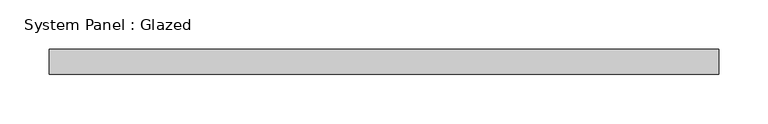
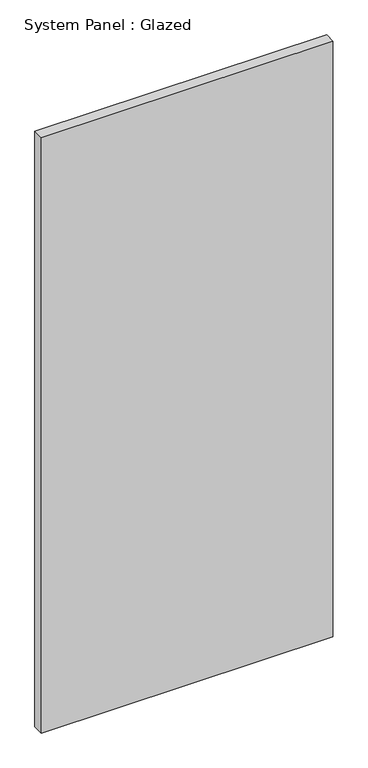
"""IFC4 building model written with IfcOpenShell, lengths in millimetres: plate geometry, System Panel : Glazed."""

from ifc_helpers import new_model, si_unit, origin, origin_with_axes, place, context, project, spatial, polyline, outline, extrude, source, transform, mapped, element, save


def system_panel_glazed_bf6811db(model_context):
    return source(origin(), model_context, "Body", "SweptSolid", [
        extrude(outline(polyline([(339.725, 19.05), (-339.725, 19.05), (-339.725, 44.45), (339.725, 44.45), (339.725, 19.05)])), origin_with_axes(), (0.0, 0.0, 1.0), 1466.2699234),
    ])


if __name__ == "__main__":
    model = new_model("IFC4")
    model_context = context("Model", 3, world=origin())
    ifc_project = project(units=[si_unit("LENGTHUNIT", "METRE", prefix="MILLI")], contexts=[model_context])
    site = spatial("IfcSite", under=ifc_project)
    building = spatial("IfcBuilding", under=site)
    placement = place(None, origin())
    system_panel_glazed_shape = system_panel_glazed_bf6811db(model_context)
    element("IfcPlate", 1, ObjectType="System Panel : Glazed", at=placement, inside=building, context=model_context, shape_type="MappedRepresentation", body=[
        mapped(system_panel_glazed_shape, transform((0.0, 0.0, 0.0), x_axis=(1.0, 0.0, 0.0), y_axis=(0.0, 1.0, 0.0), z_axis=(0.0, 0.0, 1.0))),
    ])
    save(model, "model.ifc")

# Revit data of these elements
# Type "System Panel : Glazed"
#   Construction Type Id = "GSP4R"
#   Analytic Construction = "1/8 in Pilkington single glazing"
#   Visual Light Transmittance = 0.9
#   Solar Heat Gain Coefficient = 0.86
#   Heat Transfer Coefficient (U) = 1.18115 BTU/(h·ft²·°F)
#   Define Thermal Properties by = 1
# Element 1 (IfcPlate, "System Panel : Glazed")
#   Materials on its faces: "Glass"
# Materials
#   "Glass": class "Glass", colour RGB 0 128 192, transparency 0.75, Description = "Soda Lime Glass", Cost = 0
